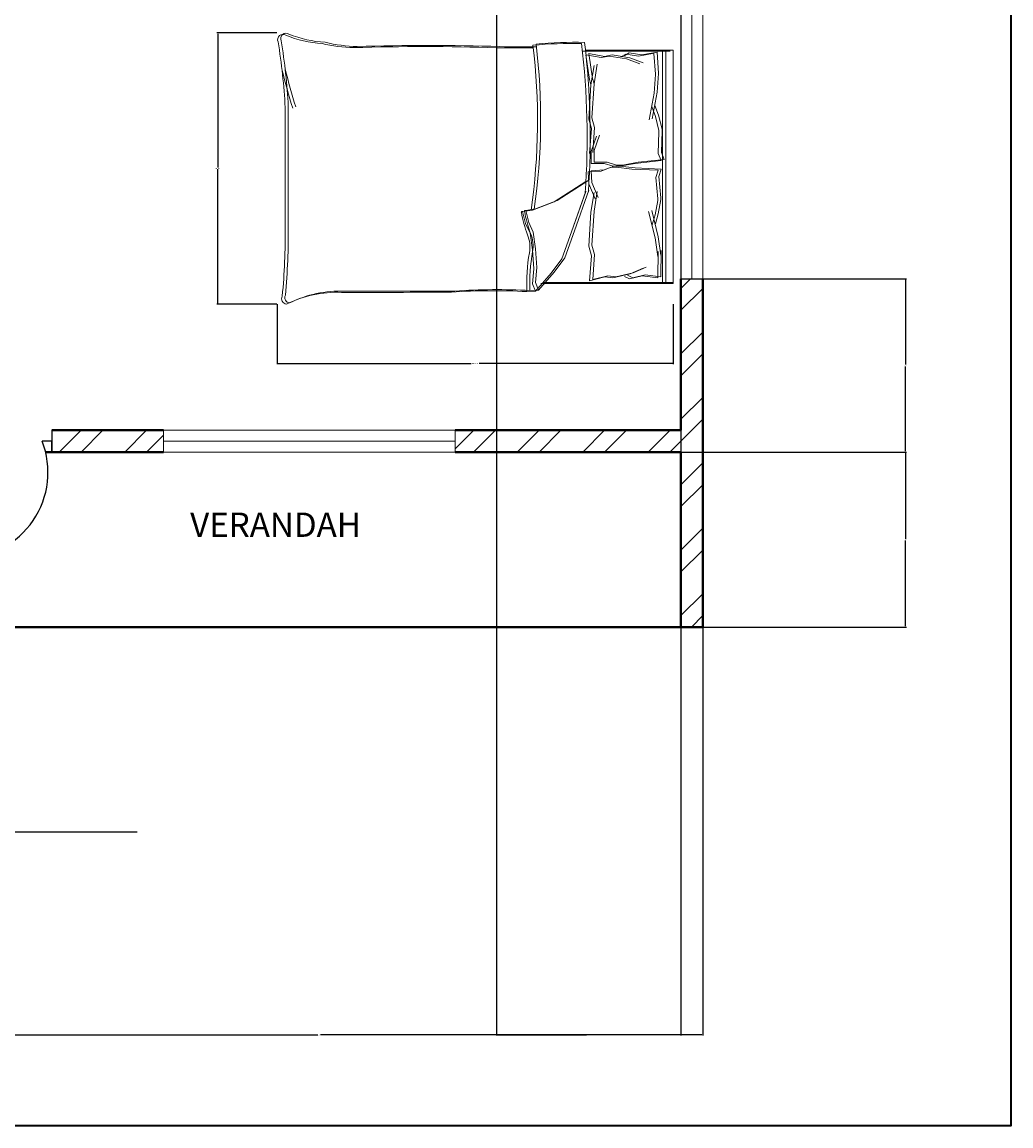
# Model space of a CAD drawing. Units: inches. Extents: x 2063 to 2617, y 1299 to 2210.
# Tile 4 of 22: x 2414 to 2617, y 1299 to 1526. Entities that reach past the tile are written whole.
import ezdxf

# ---------------------------------------------------------------- set-up
doc = ezdxf.new("R2010")
doc.units = ezdxf.units.IN
for name, color, linetype, lineweight in [('A-ANNO-DIMS', 2, 'Continuous', 18), ('A-ANNO-TEXT', 7, 'Continuous', 25), ('A-ANNO-TTLB', 7, 'Continuous', 35), ('A-AREA-IDEN', 7, 'Continuous', 18), ('A-DOOR', 11, 'Continuous', 25), ('A-FURN', 8, 'Continuous', 18), ('A-GLAZ', 123, 'Continuous', 18), ('A-WALL', 7, 'Continuous', 40)]:
    doc.layers.add(name, color=color, linetype=linetype, lineweight=lineweight)
doc.layers.add('A-WALL-PATT', color=215, linetype='Continuous', lineweight=13, true_color=0xa953a0)
doc.styles.get("Standard").update_dxf_attribs({"font": 'arial.ttf'})
doc.dimstyles.get("Standard").update_dxf_attribs({"dimtxt": 0.18, "dimasz": 0.18, "dimexe": 0.18, "dimexo": 0.0625, "dimgap": 0.09, "dimtad": 0, "dimtih": 1, "dimtoh": 1, "dimdec": 4, "dimzin": 0, "dimdsep": 46, "dimtxsty": 'Standard', "dimcen": 0.09, "dimadec": 0, "dimazin": 0, "dimtfac": 1, "dimtdec": 4, "dimtofl": 0, "dimtmove": 0, "dimatfit": 3, "dimfxl": 1, "dimtolj": 1, "dimtzin": 0, "dimarcsym": 0})

# ---------------------------------------------------------------- blocks, each defined once
blk = doc.blocks.new('BED-DOUBLE')
for p, q in [((3.48, 63.33), (3.48, 81.44)), ((3.48, 63.33), (3.48, 81.44)), ((3.48, 81.44), (51.49, 81.44)), ((3.48, 79.91), (51.27, 79.91)), ((3.48, 79.91), (51.27, 79.91)), ((3.7, 62.69), (3.7, 80.8)), ((3.7, 62.69), (3.7, 80.8)), ((24.54, 79), (25.98, 79.57)), ((24.54, 79), (25.98, 79.57)), ((25.98, 79.57), (26.56, 74.22)), ((25.98, 79.57), (26.56, 74.22)), ((51.27, 81.44), (51.27, 54.83)), ((51.27, 81.44), (51.27, 54.83)), ((51.49, 81.44), (51.49, 80.8)), ((51.49, 80.8), (51.49, 54.19)), ((51.49, 80.8), (51.49, 54.19)), ((3.7, 79.27), (51.49, 79.27)), ((3.7, 79.27), (51.49, 79.27)), ((3.89, 78.13), (4.47, 74.95)), ((3.9, 78.11), (8.18, 78.43)), ((3.9, 78.11), (8.18, 78.43)), ((3.9, 78.13), (4.47, 74.95)), ((4.12, 77.49), (4.7, 74.31)), ((4.12, 77.49), (4.7, 74.31)), ((4.13, 77.47), (8.41, 77.8)), ((4.13, 77.47), (8.41, 77.8)), ((8.18, 78.43), (8.29, 78.42)), ((8.18, 78.43), (8.29, 78.42)), ((8.29, 78.42), (12.11, 78.13)), ((8.29, 78.42), (12.11, 78.13)), ((8.41, 77.8), (8.51, 77.78)), ((8.41, 77.8), (8.51, 77.78)), ((8.51, 77.78), (12.34, 77.49)), ((8.51, 77.78), (12.34, 77.49)), ((12.11, 78.13), (17.6, 77.12)), ((12.11, 78.13), (17.6, 77.12)), ((12.34, 77.49), (17.83, 76.48)), ((12.34, 77.49), (17.83, 76.48)), ((14.86, 77.69), (16.88, 78.42)), ((14.86, 77.69), (16.88, 78.42)), ((15.08, 77.05), (17.11, 77.78)), ((15.08, 77.05), (17.11, 77.78)), ((16.88, 78.42), (19.77, 79.14)), ((16.88, 78.42), (19.77, 79.14)), ((17.11, 77.78), (20, 78.5)), ((17.11, 77.78), (20, 78.5)), ((19.77, 79.14), (20.09, 79.14)), ((19.77, 79.14), (20.09, 79.14)), ((20, 78.5), (20.32, 78.5)), ((20, 78.5), (20.32, 78.5)), ((20.09, 79.14), (24.54, 79)), ((20.09, 79.14), (24.54, 79)), ((20.32, 78.5), (24.77, 78.36)), ((20.32, 78.5), (24.77, 78.36)), ((24.77, 78.36), (26.21, 78.93)), ((24.77, 78.36), (26.21, 78.93)), ((26.21, 78.93), (26.79, 73.58)), ((26.21, 78.93), (26.79, 73.58)), ((27.98, 78.95), (27.73, 73.58)), ((27.98, 78.95), (27.73, 73.58)), ((28.21, 78.31), (27.96, 72.94)), ((28.21, 78.31), (27.96, 72.94)), ((29.46, 78.46), (27.98, 78.95)), ((29.46, 78.46), (27.98, 78.95)), ((29.68, 77.83), (28.21, 78.31)), ((29.68, 77.83), (28.21, 78.31)), ((33.88, 78.89), (29.46, 78.46)), ((33.88, 78.89), (29.46, 78.46)), ((34.11, 78.25), (29.68, 77.83)), ((34.11, 78.25), (29.68, 77.83)), ((34.21, 78.91), (33.88, 78.89)), ((34.2, 78.91), (33.88, 78.89)), ((34.43, 78.27), (34.11, 78.25)), ((34.43, 78.27), (34.11, 78.25)), ((37.14, 78.37), (34.2, 78.91)), ((37.14, 78.37), (34.21, 78.91)), ((37.36, 77.73), (34.43, 78.27)), ((37.36, 77.73), (34.43, 78.27)), ((41.91, 78.37), (36.5, 77.02)), ((41.91, 78.37), (36.5, 77.02)), ((42.14, 77.73), (36.72, 76.38)), ((42.14, 77.73), (36.72, 76.38)), ((39.2, 77.77), (37.14, 78.37)), ((39.2, 77.77), (37.14, 78.37)), ((39.43, 77.13), (37.36, 77.73)), ((39.43, 77.13), (37.36, 77.73)), ((45.71, 78.9), (41.91, 78.37)), ((45.71, 78.9), (41.91, 78.37)), ((45.94, 78.26), (42.14, 77.73)), ((45.94, 78.26), (42.14, 77.73)), ((50.11, 78.89), (44.71, 78.98)), ((44.71, 78.98), (45.71, 78.9)), ((50.11, 78.89), (44.71, 78.98)), ((44.71, 78.98), (45.71, 78.9)), ((50.34, 78.25), (44.94, 78.34)), ((44.94, 78.34), (45.94, 78.26)), ((50.34, 78.25), (44.94, 78.34)), ((44.94, 78.34), (45.94, 78.26)), ((50.11, 78.89), (49.73, 75.68)), ((50.11, 78.89), (49.73, 75.68)), ((50.34, 78.25), (49.96, 75.04)), ((50.34, 78.25), (49.96, 75.04)), ((5.05, 72.49), (6.06, 75.24)), ((5.05, 72.49), (6.06, 75.24)), ((49.31, 73.19), (48.13, 75.87)), ((49.31, 73.19), (48.13, 75.87)), ((49.54, 72.55), (48.36, 75.23)), ((49.54, 72.55), (48.36, 75.23)), ((49.73, 75.68), (50.33, 73.11)), ((49.73, 75.68), (50.33, 73.11)), ((49.96, 75.04), (50.56, 72.47)), ((49.96, 75.04), (50.56, 72.47)), ((4.47, 74.95), (4.04, 72.34)), ((4.47, 74.95), (4.04, 72.34)), ((4.7, 74.31), (4.27, 71.7)), ((4.7, 74.31), (4.27, 71.7)), ((5.28, 71.85), (6.29, 74.6)), ((5.28, 71.85), (6.29, 74.6)), ((26.56, 74.22), (27.14, 71.04)), ((26.56, 74.22), (27.14, 71.04)), ((26.79, 73.58), (27.37, 70.4)), ((26.79, 73.58), (27.37, 70.4)), ((27.73, 73.58), (27.36, 70.37)), ((27.73, 73.58), (27.36, 70.37)), ((27.96, 72.94), (27.58, 69.73)), ((27.96, 72.94), (27.58, 69.73)), ((50.11, 69.61), (49.31, 73.19)), ((50.11, 69.61), (49.31, 73.19)), ((50.33, 73.11), (49.81, 72.06)), ((50.33, 73.11), (49.82, 72.06)), ((4.04, 72.34), (4.62, 71.33)), ((4.04, 72.34), (4.62, 71.33)), ((4.27, 71.7), (4.85, 70.69)), ((4.27, 71.7), (4.85, 70.69)), ((4.47, 68.87), (5.05, 72.49)), ((4.47, 68.87), (5.05, 72.49)), ((4.7, 68.23), (5.28, 71.85)), ((4.7, 68.23), (5.28, 71.85)), ((27.14, 71.04), (27.14, 69.74)), ((27.14, 71.04), (27.14, 69.74)), ((50.34, 68.98), (49.54, 72.55)), ((50.34, 68.98), (49.54, 72.55)), ((50.56, 72.47), (50.04, 71.42)), ((50.56, 72.47), (50.04, 71.42)), ((4.76, 67.28), (4.47, 68.87)), ((4.76, 67.28), (4.47, 68.87)), ((4.99, 66.64), (4.7, 68.23)), ((4.99, 66.64), (4.7, 68.23)), ((27.14, 69.74), (26.56, 67.86)), ((27.14, 69.74), (26.56, 67.86)), ((27.37, 69.1), (26.79, 67.22)), ((27.37, 69.1), (26.79, 67.22)), ((27.36, 70.37), (27.44, 69.07)), ((27.36, 70.37), (27.44, 69.07)), ((27.37, 70.4), (27.37, 69.1)), ((27.37, 70.4), (27.37, 69.1)), ((27.44, 69.07), (28.13, 67.23)), ((27.44, 69.07), (28.13, 67.23)), ((27.58, 69.73), (27.66, 68.43)), ((27.58, 69.73), (27.66, 68.43)), ((27.66, 68.43), (28.36, 66.59)), ((27.66, 68.43), (28.36, 66.59)), ((49.92, 68.01), (50.11, 69.61)), ((49.92, 68.01), (50.11, 69.61)), ((50.15, 67.37), (50.34, 68.98)), ((50.15, 67.37), (50.34, 68.98)), ((4.18, 64.1), (4.76, 67.28)), ((4.18, 64.1), (4.76, 67.28)), ((4.41, 63.46), (4.99, 66.64)), ((4.41, 63.46), (4.99, 66.64)), ((24.1, 65.18), (20.96, 66.27)), ((24.1, 65.18), (20.96, 66.27)), ((26.56, 67.86), (26.56, 65.18)), ((26.56, 67.86), (26.56, 65.18)), ((26.79, 67.22), (26.79, 64.54)), ((26.79, 67.22), (26.79, 64.54)), ((28.13, 67.23), (28.3, 64.55)), ((28.13, 67.23), (28.3, 64.55)), ((28.36, 66.59), (28.53, 63.91)), ((28.36, 66.59), (28.53, 63.91)), ((30.75, 64.7), (33.82, 65.99)), ((30.75, 64.7), (33.82, 65.99)), ((50.7, 64.87), (49.92, 68.01)), ((50.7, 64.87), (49.92, 68.01)), ((50.93, 64.23), (50.15, 67.37)), ((50.93, 64.23), (50.15, 67.37)), ((9.28, 64.83), (4.18, 64.1)), ((9.28, 64.83), (4.18, 64.1)), ((9.51, 64.19), (4.41, 63.46)), ((9.51, 64.19), (4.41, 63.46)), ((6.38, 65.82), (10.41, 65.15)), ((6.38, 65.82), (10.41, 65.15)), ((6.61, 65.18), (10.64, 64.51)), ((6.61, 65.18), (10.64, 64.51)), ((10.41, 65.15), (9.28, 64.83)), ((10.41, 65.15), (9.28, 64.83)), ((10.64, 64.51), (9.51, 64.19)), ((10.64, 64.51), (9.51, 64.19)), ((10.41, 65.15), (17.42, 64.72)), ((10.41, 65.15), (17.42, 64.72)), ((10.64, 64.51), (17.65, 64.08)), ((10.64, 64.51), (17.65, 64.08)), ((17.42, 64.72), (19.38, 65.27)), ((17.42, 64.72), (19.38, 65.27)), ((17.65, 64.08), (19.61, 64.64)), ((17.65, 64.08), (19.61, 64.64)), ((19.38, 65.27), (24.52, 64.87)), ((19.38, 65.27), (24.52, 64.87)), ((19.61, 64.64), (24.74, 64.23)), ((19.61, 64.64), (24.74, 64.23)), ((24.33, 64.54), (21.19, 65.63)), ((24.33, 64.54), (21.19, 65.63)), ((26.56, 65.18), (24.1, 65.18)), ((26.56, 65.18), (24.1, 65.18)), ((26.79, 64.54), (24.33, 64.54)), ((26.79, 64.54), (24.33, 64.54)), ((28.3, 64.55), (30.75, 64.7)), ((28.3, 64.55), (30.75, 64.7)), ((28.53, 63.91), (30.98, 64.06)), ((28.53, 63.91), (30.98, 64.06)), ((30.26, 64.06), (34.45, 57.57)), ((30.26, 64.06), (34.45, 57.57)), ((30.98, 64.06), (34.05, 65.35)), ((30.98, 64.06), (34.05, 65.35)), ((40.64, 61.13), (32.31, 64.06)), ((40.64, 61.13), (32.31, 64.06)), ((32.56, 65.82), (36.6, 65.15)), ((32.56, 65.82), (36.6, 65.15)), ((32.79, 65.18), (36.83, 64.51)), ((32.79, 65.18), (36.82, 64.51)), ((36.6, 65.15), (43.61, 64.72)), ((36.6, 65.15), (43.61, 64.72)), ((36.82, 64.51), (43.83, 64.08)), ((36.83, 64.51), (43.84, 64.08)), ((43.61, 64.72), (45.57, 65.27)), ((43.61, 64.72), (45.57, 65.27)), ((43.83, 64.08), (45.8, 64.64)), ((43.84, 64.08), (45.8, 64.64)), ((45.57, 65.27), (50.7, 64.87)), ((45.57, 65.27), (50.7, 64.87)), ((45.8, 64.64), (50.93, 64.23)), ((45.8, 64.64), (50.93, 64.23)), ((30.49, 63.42), (34.68, 56.93)), ((30.49, 63.42), (34.68, 56.93)), ((40.87, 60.49), (32.53, 63.42)), ((40.87, 60.49), (32.54, 63.42)), ((46.22, 59.11), (40.64, 61.13)), ((46.22, 59.11), (40.64, 61.13)), ((46.45, 58.48), (40.87, 60.49)), ((46.45, 58.48), (40.87, 60.49)), ((49.16, 56.95), (46.22, 59.11)), ((49.16, 56.95), (46.22, 59.11)), ((34.45, 57.57), (36.15, 53.08)), ((34.45, 57.57), (36.15, 53.08)), ((34.68, 56.93), (36.38, 52.44)), ((34.68, 56.93), (36.38, 52.44)), ((49.39, 56.31), (46.45, 58.48)), ((49.39, 56.31), (46.45, 58.48)), ((52.87, 53.7), (49.16, 56.95)), ((52.87, 53.7), (49.16, 56.95)), ((53.1, 53.06), (49.39, 56.31)), ((53.1, 53.06), (49.39, 56.31)), ((36.15, 53.08), (36.46, 51.07)), ((36.15, 53.08), (36.46, 51.07)), ((36.38, 52.44), (36.69, 50.43)), ((36.38, 52.44), (36.69, 50.43)), ((38.94, 51.69), (40.95, 52.61)), ((38.94, 51.69), (40.95, 52.61)), ((40.95, 52.61), (44.36, 53.08)), ((40.95, 52.61), (44.36, 53.08)), ((41.18, 51.97), (44.59, 52.44)), ((41.18, 51.97), (44.59, 52.44)), ((44.36, 53.08), (48.23, 53.39)), ((44.36, 53.08), (48.23, 53.39)), ((44.59, 52.44), (48.46, 52.75)), ((44.59, 52.44), (48.46, 52.75)), ((48.23, 53.39), (51.33, 53.08)), ((48.23, 53.39), (51.33, 53.08)), ((48.46, 52.75), (51.56, 52.44)), ((48.46, 52.75), (51.56, 52.44)), ((51.33, 53.08), (52.87, 53.7)), ((51.33, 53.08), (52.87, 53.7)), ((51.56, 52.44), (53.1, 53.06)), ((51.56, 52.44), (53.1, 53.06)), ((52.95, 51.95), (52.87, 53.7, 3.87)), ((52.95, 51.95), (52.87, 53.7, 3.87)), ((53.18, 51.31), (53.1, 53.06, 3.87)), ((53.18, 51.31), (53.1, 53.06, 3.87)), ((36.46, 51.07), (38.94, 51.69)), ((36.46, 51.07), (38.94, 51.69)), ((36.69, 50.43), (39.17, 51.05)), ((36.69, 50.43), (39.17, 51.05)), ((39.17, 51.05), (41.18, 51.97)), ((39.17, 51.05), (41.18, 51.97)), ((15.06, 2.2), (39.68, 2.2)), ((15.06, 2.2), (39.68, 2.2)), ((15.29, 1.56), (39.91, 1.56)), ((15.29, 1.56), (39.91, 1.56))]:
    blk.add_line(p, q)
for centre, radius, start, end in [((21.36, -100.61), 164.97, 86.0865, 96.7821), ((21.36, -100.61), 164.97, 86.0865, 96.7821), ((21.59, -101.25), 164.97, 86.0865, 96.7821), ((21.59, -101.25), 164.97, 86.0865, 96.7821), ((85.16, 61.35), 83.31, 178.7218, 185.604), ((85.16, 61.35), 83.31, 178.7218, 185.604), ((85.39, 60.71), 83.31, 178.7218, 185.604), ((85.39, 60.71), 83.31, 178.7218, 185.604), ((17.76, -74.87), 129.02, 81.7845, 96.9006), ((17.76, -74.87), 129.02, 81.7845, 96.9006), ((17.98, -75.51), 129.02, 81.7845, 96.9006), ((17.98, -75.51), 129.02, 81.7845, 96.9006), ((-167.31, 50.27), 170.11, 358.4762, 1.0082), ((-167.31, 50.27), 170.11, 358.4762, 1.0082), ((-167.08, 49.63), 170.11, 358.4762, 1.0082), ((-167.08, 49.63), 170.11, 358.4762, 1.0082), ((43.74, 46.38), 6.22, 78.6608, 113.7384), ((43.74, 46.38), 6.22, 78.6608, 113.7384), ((51.33, 88.1), 36.18, 259.8763, 272.5657), ((51.33, 88.1), 36.18, 259.8763, 272.5657), ((36.64, 51), 0.185, 160.2464, 271.1377), ((36.64, 51), 0.185, 160.2464, 271.1377), ((31.15, 79.96), 29.65, 280.6617, 289.8806), ((31.15, 79.96), 29.65, 280.6617, 289.8806), ((36.87, 50.36), 0.185, 160.2464, 271.1377), ((36.86, 50.36), 0.185, 160.2464, 271.1377), ((31.38, 79.32), 29.65, 280.6617, 289.8806), ((31.38, 79.32), 29.65, 280.6617, 289.8806), ((43.97, 45.74), 6.22, 78.6608, 113.7384), ((43.97, 45.74), 6.22, 78.6608, 113.7384), ((51.56, 87.46), 36.18, 259.8763, 272.5657), ((51.56, 87.46), 36.18, 259.8763, 272.5657), ((182.27, 45.13), 129.5, 176.9791, 183.8365), ((182.27, 45.13), 129.5, 176.9791, 183.8365), ((182.49, 44.49), 129.5, 176.9791, 183.8365), ((182.49, 44.49), 129.5, 176.9791, 183.8365), ((484.82, 30.83), 482.31, 178.2277, 181.7185), ((484.82, 30.83), 482.31, 178.2277, 181.7185), ((485.05, 30.19), 482.31, 178.2277, 181.7185), ((485.05, 30.19), 482.31, 178.2277, 181.7185), ((-4508.74, 13.62), 4561.86, 0.00217, 0.28689), ((-4508.74, 13.62), 4561.86, 0.00217, 0.28689), ((-4508.51, 12.98), 4561.86, 0.00217, 0.28689), ((-4508.51, 12.98), 4561.86, 0.00217, 0.28689), ((-26.9, 16.93), 29.63, 346.0648, 358.9113), ((-26.9, 16.93), 29.63, 346.0648, 358.9113), ((-26.67, 16.29), 29.63, 346.0648, 358.9113), ((-26.67, 16.29), 29.63, 346.0648, 358.9113), ((76.16, 12.78), 23.07, 177.4714, 206.4681), ((76.16, 12.78), 23.07, 177.4714, 206.4681), ((76.39, 12.14), 23.07, 177.4714, 206.4681), ((76.39, 12.14), 23.07, 177.4714, 206.4681), ((-21.66, 11.17), 23.56, 337.9751, 356.652), ((-21.66, 11.17), 23.56, 337.9751, 356.652), ((-21.43, 10.53), 23.56, 337.9751, 356.652), ((-21.43, 10.53), 23.56, 337.9751, 356.652), ((1.09, 1.73), 1.09, 146.1736, 293.4781), ((1.09, 1.73), 1.09, 146.1736, 293.4781), ((-17.22, 105.16), 106.46, 283.3832, 287.7053), ((-17.22, 105.16), 106.46, 283.3832, 287.7053), ((-16.99, 104.52), 106.46, 283.3832, 287.7053), ((-16.99, 104.52), 106.46, 283.3832, 287.7053), ((54.41, 2.57), 1.1, 242.6588, 356.02), ((54.41, 2.57), 1.1, 242.6588, 356.02), ((1.32, 1.09), 1.09, 146.1736, 293.4781), ((1.32, 1.09), 1.09, 146.1736, 293.4781), ((21.43, -119.39), 121.76, 92.9958, 99.4091), ((21.43, -119.39), 121.76, 92.9958, 99.4091), ((21.66, -120.03), 121.76, 92.9958, 99.4091), ((21.66, -120.03), 121.76, 92.9958, 99.4091), ((41.15, -130.83), 133.04, 84.4998, 90.6351), ((41.15, -130.83), 133.04, 84.4998, 90.6351), ((41.38, -131.47), 133.04, 84.4998, 90.6351), ((41.38, -131.47), 133.04, 84.4998, 90.6351), ((54.64, 1.93), 1.1, 242.6588, 356.02), ((54.64, 1.93), 1.1, 242.6588, 356.02)]:
    blk.add_arc(centre, radius, start, end)
blk = doc.blocks.new('WIN-60IN')
for p, q in [((0, 60), (4.5, 60)), ((0, 60), (0, 0)), ((4.5, 60), (2.25, 60)), ((2.25, 60), (2.25, 0)), ((4.5, 60), (4.5, 0)), ((2.25, 0), (0, 0)), ((0, 0), (4.5, 0))]:
    blk.add_line(p, q)
blk = doc.blocks.new('*D13')
at = {"layer": 'A-ANNO-DIMS', "color": 0, "lineweight": -2, "transparency": 16777216}
for p, q in [((2466, 1468.24), (2466, 1455.89)), ((2547.55, 1468.24), (2547.55, 1455.89)), ((2466.18, 1456.07), (2505.95, 1456.07)), ((2547.37, 1456.07), (2507.59, 1456.07))]:
    blk.add_line(p, q, dxfattribs=at)
at = {"layer": 'A-ANNO-DIMS', "color": 0, "transparency": 16777216}
for points in [[(2466.18, 1456.1), (2466.18, 1456.04), (2466, 1456.07)], [(2547.37, 1456.1), (2547.37, 1456.04), (2547.55, 1456.07)]]:
    blk.add_solid(points, dxfattribs=at)
at = {"layer": 'Defpoints', "color": 0, "transparency": 16777216}
for p in [(2466, 1468.3), (2547.55, 1468.3), (2547.55, 1456.07)]:
    blk.add_point(p, dxfattribs=at)
at = {"layer": 'A-ANNO-DIMS', "color": 0, "transparency": 16777216, "insert": (2506.77, 1456.07), "char_height": 0.18, "attachment_point": 5}
blk.add_mtext('\\A1;BED 82 TYP.', dxfattribs=at)
blk = doc.blocks.new('*D14')
at = {"layer": 'A-ANNO-DIMS', "color": 0, "lineweight": -2, "transparency": 16777216}
for p, q in [((2465.94, 1524.12), (2453.59, 1524.12)), ((2453.77, 1523.94), (2453.77, 1496.39)), ((2453.77, 1468.48), (2453.77, 1496.03)), ((2465.94, 1468.3), (2453.59, 1468.3))]:
    blk.add_line(p, q, dxfattribs=at)
at = {"layer": 'A-ANNO-DIMS', "color": 0, "transparency": 16777216}
for points in [[(2453.74, 1523.94), (2453.8, 1523.94), (2453.77, 1524.12)], [(2453.74, 1468.48), (2453.8, 1468.48), (2453.77, 1468.3)]]:
    blk.add_solid(points, dxfattribs=at)
at = {"layer": 'Defpoints', "color": 0, "transparency": 16777216}
for p in [(2466, 1524.12), (2453.77, 1468.3), (2466, 1468.3)]:
    blk.add_point(p, dxfattribs=at)
at = {"layer": 'A-ANNO-DIMS', "color": 0, "transparency": 16777216, "insert": (2453.77, 1496.21), "char_height": 0.18, "attachment_point": 5}
blk.add_mtext('\\A1;56 TYP.', dxfattribs=at)
blk = doc.blocks.new('*D35')
at = {"layer": 'A-ANNO-DIMS', "color": 0, "lineweight": -2, "transparency": 16777216}
for p, q in [((2395.64, 1401.75), (2395.64, 1317.7)), ((2553.64, 1401.75), (2553.64, 1317.7)), ((2395.82, 1317.88), (2474.36, 1317.88)), ((2553.46, 1317.88), (2474.92, 1317.88))]:
    blk.add_line(p, q, dxfattribs=at)
at = {"layer": 'A-ANNO-DIMS', "color": 0, "transparency": 16777216}
for points in [[(2395.82, 1317.91), (2395.82, 1317.85), (2395.64, 1317.88)], [(2553.46, 1317.91), (2553.46, 1317.85), (2553.64, 1317.88)]]:
    blk.add_solid(points, dxfattribs=at)
at = {"layer": 'Defpoints', "color": 0, "transparency": 16777216}
for p in [(2395.64, 1401.81), (2553.64, 1401.81), (2553.64, 1317.88)]:
    blk.add_point(p, dxfattribs=at)
at = {"layer": 'A-ANNO-DIMS', "color": 0, "transparency": 16777216, "insert": (2474.64, 1317.88), "char_height": 0.18, "attachment_point": 5}
blk.add_mtext('\\A1;158', dxfattribs=at)
blk = doc.blocks.new('*D36')
at = {"layer": 'A-ANNO-DIMS', "color": 0, "lineweight": -2, "transparency": 16777216}
for p, q in [((2549.21, 1437.81), (2595.57, 1437.81)), ((2595.39, 1437.63), (2595.39, 1419.99)), ((2595.39, 1401.99), (2595.39, 1419.63)), ((2549.21, 1401.81), (2595.57, 1401.81))]:
    blk.add_line(p, q, dxfattribs=at)
at = {"layer": 'A-ANNO-DIMS', "color": 0, "transparency": 16777216}
for points in [[(2595.36, 1437.63), (2595.42, 1437.63), (2595.39, 1437.81)], [(2595.36, 1401.99), (2595.42, 1401.99), (2595.39, 1401.81)]]:
    blk.add_solid(points, dxfattribs=at)
at = {"layer": 'Defpoints', "color": 0, "transparency": 16777216}
for p in [(2549.14, 1437.81), (2595.39, 1437.81), (2549.14, 1401.81)]:
    blk.add_point(p, dxfattribs=at)
at = {"layer": 'A-ANNO-DIMS', "color": 0, "transparency": 16777216, "insert": (2595.39, 1419.81), "char_height": 0.18, "attachment_point": 5}
blk.add_mtext('\\A1;36', dxfattribs=at)
blk = doc.blocks.new('*D37')
at = {"layer": 'A-ANNO-DIMS', "color": 0, "lineweight": -2, "transparency": 16777216}
for p, q in [((2549.21, 1473.48), (2595.57, 1473.48)), ((2595.39, 1473.3), (2595.39, 1455.83)), ((2595.39, 1437.99), (2595.39, 1455.46)), ((2549.21, 1437.81), (2595.57, 1437.81))]:
    blk.add_line(p, q, dxfattribs=at)
at = {"layer": 'A-ANNO-DIMS', "color": 0, "transparency": 16777216}
for points in [[(2595.36, 1473.3), (2595.42, 1473.3), (2595.39, 1473.48)], [(2595.36, 1437.99), (2595.42, 1437.99), (2595.39, 1437.81)]]:
    blk.add_solid(points, dxfattribs=at)
at = {"layer": 'Defpoints', "color": 0, "transparency": 16777216}
for p in [(2549.14, 1473.48), (2595.39, 1473.48), (2549.14, 1437.81)]:
    blk.add_point(p, dxfattribs=at)
at = {"layer": 'A-ANNO-DIMS', "color": 0, "transparency": 16777216, "insert": (2595.39, 1455.65), "char_height": 0.18, "attachment_point": 5}
blk.add_mtext('\\A1;35.67', dxfattribs=at)
blk = doc.blocks.new('*D52')
at = {"layer": 'A-ANNO-DIMS', "color": 0, "lineweight": -2, "transparency": 16777216}
for p, q in [((2511.17, 2124.25), (2511.17, 1317.7)), ((2549.14, 2124.25), (2549.14, 1317.7)), ((2511.35, 1317.88), (2529.69, 1317.88)), ((2548.96, 1317.88), (2530.62, 1317.88))]:
    blk.add_line(p, q, dxfattribs=at)
at = {"layer": 'A-ANNO-DIMS', "color": 0, "transparency": 16777216}
for points in [[(2511.35, 1317.91), (2511.35, 1317.85), (2511.17, 1317.88)], [(2548.96, 1317.91), (2548.96, 1317.85), (2549.14, 1317.88)]]:
    blk.add_solid(points, dxfattribs=at)
at = {"layer": 'Defpoints', "color": 0, "transparency": 16777216}
for p in [(2511.17, 2124.31), (2549.14, 2124.31), (2549.14, 1317.88)]:
    blk.add_point(p, dxfattribs=at)
at = {"layer": 'A-ANNO-DIMS', "color": 0, "transparency": 16777216, "insert": (2530.16, 1317.88), "char_height": 0.18, "attachment_point": 5}
blk.add_mtext('\\A1;37.974', dxfattribs=at)

msp = doc.modelspace()

# ---------------------------------------------------------------- hatches: boundary and pattern name
at = {"layer": 'A-WALL-PATT'}
h = msp.add_hatch(dxfattribs=at)
h.set_pattern_fill('ANSI32', color=256)
h.paths.add_polyline_path([(2553.6442, 2128.8122), (2511.1703, 2128.8122), (2511.1703, 2124.3122), (2549.1442, 2124.3122), (2549.1442, 2095.662), (2553.6442, 2095.662)])
h.paths.add_polyline_path([(2553.6442, 2035.662), (2549.1442, 2035.662), (2549.1442, 1980.3122), (2503.7214, 1980.3122), (2503.7214, 1975.8122), (2549.1442, 1975.8122), (2549.1442, 1962.9693), (2553.6442, 1962.9693)])
h.paths.add_polyline_path([(2553.6442, 1938.9693), (2549.1442, 1938.9693), (2549.1442, 1927.8122), (2477.1442, 1927.8122), (2477.1442, 1975.8122), (2481.2918, 1975.8122), (2481.2918, 1980.3122), (2453.2648, 1980.3122), (2453.2648, 1975.8122), (2472.6442, 1975.8122), (2472.6442, 1868.3122), (2400.6442, 1868.3122), (2400.6442, 1861.3782), (2405.1442, 1861.3782), (2405.1442, 1863.8122), (2480.9699, 1863.8122), (2480.9699, 1866.0622), (2480.9699, 1868.3122), (2477.1442, 1868.3122), (2477.1442, 1923.3122), (2549.1442, 1923.3122), (2549.1442, 1908.8504), (2553.6442, 1908.8504)])
h.paths.add_polyline_path([(2553.6442, 1884.8504), (2549.1442, 1884.8504), (2549.1442, 1868.3122), (2501.0636, 1868.3122), (2501.0636, 1863.8122), (2549.1442, 1863.8122), (2549.1442, 1826.0298), (2553.6442, 1826.0298)])
h.paths.add_polyline_path([(2388.1504, 1980.3122), (2340.6442, 1980.3122), (2340.6442, 2124.3122), (2358.7501, 2124.3122), (2358.7501, 2128.8122), (2316.3482, 2128.8122), (2316.3482, 2124.3122), (2336.1442, 2124.3122), (2336.1442, 1980.3122), (2289.1737, 1980.3122), (2289.1737, 1975.8122), (2336.1442, 1975.8122), (2336.1442, 1619.3122), (2333.1433, 1619.3122), (2333.1433, 1614.8122), (2344.1671, 1614.8122), (2344.1671, 1617.0622), (2344.1671, 1619.3122), (2340.6442, 1619.3122), (2340.6442, 1975.8122), (2388.1504, 1975.8122), (2388.1504, 1978.0622)])
h.paths.add_polyline_path([(2290.1442, 1614.8122), (2301.4594, 1614.8122), (2301.4594, 1617.0622), (2301.4594, 1619.3122), (2285.6442, 1619.3122), (2285.6442, 1566.8122), (2280.8619, 1566.8122), (2280.8619, 1564.5622), (2280.8619, 1562.3122), (2285.6442, 1562.3122), (2285.6442, 1442.3122), (2281.7879, 1442.3122), (2281.7879, 1437.8122), (2285.6442, 1437.8122), (2285.6442, 1401.8122), (2290.1442, 1401.8122)])
h.paths.add_polyline_path([(2549.1442, 1731.8122), (2405.1442, 1731.8122), (2405.1442, 1834.4638), (2402.8942, 1834.4638), (2400.6442, 1834.4638), (2400.6442, 1727.3122), (2549.1442, 1727.3122)])
h.paths.add_polyline_path([(2553.6442, 1766.0298), (2551.3942, 1766.0298), (2549.1442, 1766.0298), (2549.1442, 1686.7767), (2553.6442, 1686.7767)])
h.paths.add_polyline_path([(2553.6442, 1638.7767), (2551.3942, 1638.7767), (2549.1442, 1638.7767), (2549.1442, 1619.3122), (2448.6442, 1619.3122), (2448.6442, 1610.5671), (2450.8942, 1610.5671), (2453.1442, 1610.5671), (2453.1442, 1614.8122), (2549.1442, 1614.8122), (2549.1442, 1601.6421), (2553.6442, 1601.6421)])
h.paths.add_polyline_path([(2553.6442, 1577.6421), (2551.3942, 1577.6421), (2549.1442, 1577.6421), (2549.1442, 1566.8122), (2453.1442, 1566.8122), (2453.1442, 1591.5045), (2451.0335, 1591.5045), (2448.6442, 1591.5045), (2448.6442, 1566.8122), (2434.0475, 1566.8122), (2434.0475, 1562.3122), (2549.1442, 1562.3122), (2549.1442, 1533.48), (2553.6442, 1533.48)])
h.paths.add_polyline_path([(2553.6442, 1473.48), (2549.1442, 1473.48), (2549.1442, 1442.3122), (2502.6258, 1442.3122), (2502.6258, 1437.8122), (2549.1442, 1437.8122), (2549.1442, 1401.8122), (2553.6442, 1401.8122)])
h.paths.add_polyline_path([(2395.6442, 1562.3122), (2400.0901, 1562.3122), (2400.0901, 1564.5622), (2400.0901, 1566.8122), (2395.6442, 1566.8122), (2395.6442, 1619.3122), (2379.1127, 1619.3122), (2379.1127, 1614.8122), (2391.1442, 1614.8122), (2391.1442, 1401.8122), (2395.6442, 1401.8122), (2395.6442, 1437.8122), (2399.2425, 1437.8122), (2399.2425, 1440.0622), (2399.2425, 1442.3122), (2395.6442, 1442.3122)])
h.paths.add_polyline_path([(2442.6258, 1442.3122), (2419.6262, 1442.3122), (2419.6262, 1437.8122), (2442.6258, 1437.8122), (2442.6258, 1440.0622)])
h.paths.add_polyline_path([(2127.6442, 1480.2532), (2125.3942, 1480.2532), (2123.1442, 1480.2532), (2123.1442, 1401.8122), (2127.6442, 1401.8122), (2127.6442, 1437.8122), (2145.1538, 1437.8122), (2145.1538, 1440.0622), (2145.1538, 1442.3122), (2127.6442, 1442.3122)])
h.paths.add_polyline_path([(2259.809, 1442.3122), (2205.1538, 1442.3122), (2205.1538, 1437.8122), (2259.809, 1437.8122), (2259.809, 1440.0622)])
h.paths.add_polyline_path([(2127.6442, 1659.7652), (2123.1442, 1659.7652), (2123.1442, 1605.5161), (2125.3942, 1605.5161), (2127.6442, 1605.5161), (2127.6442, 1614.8122), (2223.6442, 1614.8122), (2223.6442, 1611.2723), (2228.1442, 1611.2723), (2228.1442, 1619.3122), (2127.6442, 1619.3122)])
h.paths.add_polyline_path([(2244.8673, 1566.8122), (2228.1442, 1566.8122), (2228.1442, 1590.8122), (2225.8942, 1590.8122), (2223.6442, 1590.8122), (2223.6442, 1566.8122), (2127.6442, 1566.8122), (2127.6442, 1581.5161), (2123.1442, 1581.5161), (2123.1442, 1540.2532), (2127.6442, 1540.2532), (2127.6442, 1562.3122), (2244.8673, 1562.3122), (2244.8673, 1564.5622)])
h.paths.add_polyline_path([(2172.5174, 1868.3122), (2127.6442, 1868.3122), (2127.6442, 1886.5833), (2123.1442, 1886.5833), (2123.1442, 1832.6633), (2127.6442, 1832.6633), (2127.6442, 1863.8122), (2172.5174, 1863.8122), (2172.5174, 1866.0622)])
h.paths.add_polyline_path([(2276.1442, 1868.3122), (2204.1442, 1868.3122), (2204.1442, 1923.3122), (2204.1442, 1975.8122), (2224.8362, 1975.8122), (2224.8362, 1978.1097), (2224.8362, 1980.3122), (2195.0729, 1980.3122), (2195.0729, 1978.0622), (2195.0729, 1975.8122), (2199.6442, 1975.8122), (2199.6442, 1927.8122), (2127.6442, 1927.8122), (2127.6442, 1942.3492), (2123.1442, 1942.3492), (2123.1442, 1910.5833), (2127.6442, 1910.5833), (2127.6442, 1923.3122), (2199.6442, 1923.3122), (2199.6442, 1868.3122), (2194.8228, 1868.3122), (2194.8228, 1864.7337), (2194.8228, 1863.8122), (2271.6442, 1863.8122), (2271.6442, 1860.0507), (2276.1442, 1860.0507)])
h.paths.add_polyline_path([(2276.1442, 1829.994), (2273.8942, 1829.994), (2271.6442, 1829.994), (2271.6442, 1731.8122), (2127.6442, 1731.8122), (2127.6442, 1772.6633), (2123.1442, 1772.6633), (2123.1442, 1707.7652), (2127.6442, 1707.7652), (2127.6442, 1727.3122), (2276.1442, 1727.3122)])
h.paths.add_polyline_path([(2127.6442, 2022.1152), (2123.1442, 2022.1152), (2123.1442, 1966.3492), (2127.6442, 1966.3492), (2127.6442, 1975.8122), (2174.2082, 1975.8122), (2174.2082, 1978.0622), (2174.2082, 1980.3122), (2127.6442, 1980.3122)])
h.paths.add_polyline_path([(2361.9755, 1678.588), (2398.4558, 1678.588), (2398.4558, 1697.2453), (2361.9755, 1697.2453)], flags=9)
h.paths.add_polyline_path([(2351.5397, 1780.4072), (2386.1987, 1780.4072), (2386.1987, 1790.7107), (2351.5397, 1790.7107)], flags=25)
h.paths.add_polyline_path([(2350.6753, 1940.9321), (2387.6024, 1940.9321), (2387.6024, 1959.5894), (2350.6753, 1959.5894)], flags=25)
h.paths.add_polyline_path([(2254.9545, 1684.638), (2295.0943, 1684.638), (2295.0943, 1703.2953), (2254.9545, 1703.2953)], flags=9)
h.paths.add_polyline_path([(2282.4946, 1782.4438), (2317.1535, 1782.4438), (2317.1535, 1792.7474), (2282.4946, 1792.7474)], flags=9)
h.paths.add_polyline_path([(2270.327, 1939.2854), (2307.254, 1939.2854), (2307.254, 1957.9428), (2270.327, 1957.9428)], flags=9)

# ---------------------------------------------------------------- linework, layer by layer
at = {"layer": 'A-ANNO-TEXT'}
msp.add_line((2245.3388, 1359.6321), (2437.1908, 1359.6321), dxfattribs=at)
at = {"layer": 'A-ANNO-TTLB'}
msp.add_lwpolyline([(2062.5792, 2209.6485), (2617.0648, 2209.6485), (2617.0648, 1299.1125), (2062.5792, 1299.1125)], close=True, dxfattribs=at)
at = {"layer": 'A-DOOR'}
for p, q in [((2419.6262, 1442.3122), (2419.6262, 1437.8122)), ((2419.6262, 1440.0622), (2417.6262, 1440.0622)), ((2419.6262, 1437.8122), (2419.6262, 1440.0622))]:
    msp.add_line(p, q, dxfattribs=at)
msp.add_arc((2401.2425, 1433.6544), 17.5922, 270, 21.360924, dxfattribs=at)
at = {"layer": 'A-GLAZ'}
for p, q in [((2549.1442, 1533.48), (2549.1442, 1473.48)), ((2551.3942, 1533.48), (2551.3942, 1473.48)), ((2553.6442, 1533.48), (2553.6442, 1473.48)), ((2553.6442, 1473.48), (2549.1442, 1473.48)), ((2551.3942, 1473.48), (2553.6442, 1473.48))]:
    msp.add_line(p, q, dxfattribs=at)
at = {"layer": 'A-WALL'}
for p, q in [((2549.1442, 1473.48), (2549.1442, 1442.3122)), ((2553.6442, 1473.48), (2553.6442, 1401.8122)), ((2419.6262, 1442.3122), (2442.6258, 1442.3122)), ((2502.6258, 1442.3122), (2549.1442, 1442.3122)), ((2418.3363, 1437.8122), (2442.6258, 1437.8122)), ((2502.6258, 1437.8122), (2549.1442, 1437.8122)), ((2549.1442, 1437.8122), (2549.1442, 1401.8122)), ((2123.1442, 1401.8122), (2553.6442, 1401.8122))]:
    msp.add_line(p, q, dxfattribs=at)

# ---------------------------------------------------------------- block references
at = {"layer": 'A-FURN', "rotation": 270}
msp.add_blockref('BED-DOUBLE', (2466.1025, 1524.0378), dxfattribs=at)
at = {"layer": 'A-GLAZ', "extrusion": (0, 0, -1), "zscale": -1, "rotation": 90}
msp.add_blockref('WIN-60IN', (-2442.6256, 1437.8119), dxfattribs=at)

# ---------------------------------------------------------------- texts
at = {"layer": 'A-AREA-IDEN', "insert": (2448.1005, 1425.3685), "char_height": 5, "attachment_point": 1}
msp.add_mtext_dynamic_manual_height_columns('VERANDAH', width=126.284856, gutter_width=12.5, heights=[0], dxfattribs=at)

# ---------------------------------------------------------------- dimensions: what is measured, and where the dimension line sits
at = {"layer": 'A-ANNO-DIMS'}
for base, p1, p2, override, picture, middle in [((2549.1442, 1317.8821), (2511.1703, 2124.3122), (2549.1442, 2124.3122), {"dimdec": 3, "dimlfac": 1, "dimrnd": 0, "dimzin": 0, "dimdsep": 46, "dimlunit": 2}, '*D52', (2530.1573, 1317.8821)), ((2553.6442, 1317.8821), (2395.6442, 1401.8122), (2553.6442, 1401.8122), {"dimdec": 0, "dimlfac": 1, "dimrnd": 0, "dimzin": 0, "dimdsep": 46, "dimlunit": 2}, '*D35', (2474.6442, 1317.8821))]:
    dim = msp.add_linear_dim(base=base, p1=p1, p2=p2, dimstyle='Standard', override=override, dxfattribs=at)
    dim.commit()
    dim.dimension.update_dxf_attribs({"geometry": picture, "text_midpoint": middle})
dim = msp.add_linear_dim(base=(2453.7653, 1468.2992), p1=(2465.9976, 1524.1238), p2=(2465.9976, 1468.2992), angle=270, text='<> TYP.', dimstyle='Standard', override={"dimdec": 0, "dimlfac": 1, "dimrnd": 0, "dimzin": 0, "dimdsep": 46, "dimlunit": 2}, dxfattribs=at)
dim.commit()
dim.dimension.update_dxf_attribs({"geometry": '*D14', "text_midpoint": (2453.7653, 1496.2115)})
for base, p1, p2, override, picture, middle in [((2595.3943, 1473.48), (2549.1442, 1437.8122), (2549.1442, 1473.48), {"dimdec": 2, "dimlfac": 1, "dimrnd": 0, "dimzin": 0, "dimdsep": 46, "dimlunit": 2}, '*D37', (2595.3943, 1455.6461)), ((2595.3943, 1437.8122), (2549.1442, 1401.8122), (2549.1442, 1437.8122), {"dimdec": 0, "dimlfac": 1, "dimrnd": 0, "dimzin": 0, "dimdsep": 46, "dimlunit": 2}, '*D36', (2595.3943, 1419.8122))]:
    dim = msp.add_linear_dim(base=base, p1=p1, p2=p2, angle=90, dimstyle='Standard', override=override, dxfattribs=at)
    dim.commit()
    dim.dimension.update_dxf_attribs({"geometry": picture, "text_midpoint": middle})
dim = msp.add_linear_dim(base=(2547.5462, 1456.0669), p1=(2465.9976, 1468.2992), p2=(2547.5462, 1468.2992), text='BED <> TYP.', dimstyle='Standard', override={"dimdec": 0, "dimlfac": 1, "dimrnd": 0, "dimzin": 0, "dimdsep": 46, "dimlunit": 2}, dxfattribs=at)
dim.commit()
dim.dimension.update_dxf_attribs({"geometry": '*D13', "text_midpoint": (2506.7719, 1456.0669)})

doc.saveas('drawing.dxf')
